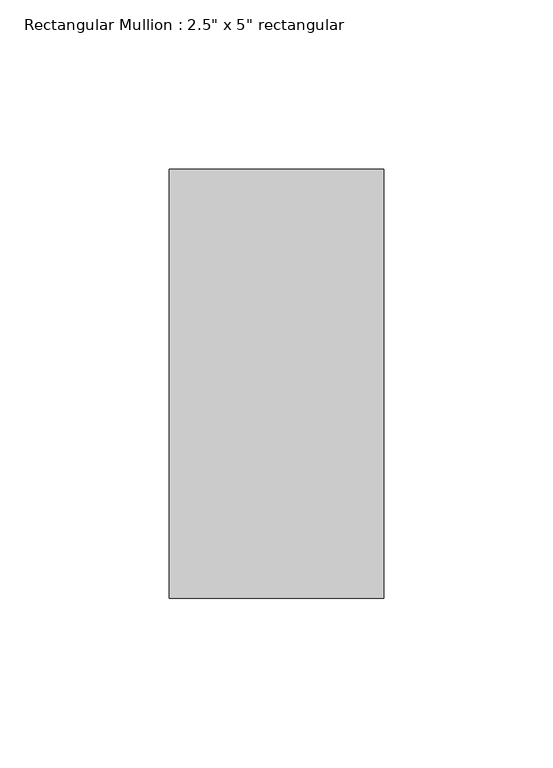
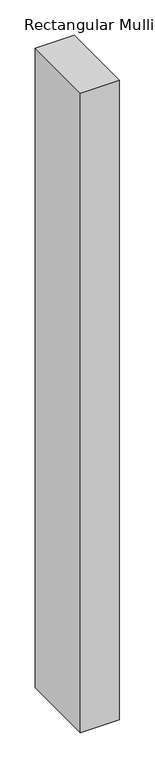
"""IFC4 building model written with IfcOpenShell, lengths in millimetres: member geometry."""

from ifc_helpers import new_model, si_unit, frame, origin, place, context, project, spatial, polyline, outline, extrude, source, transform, mapped, element, save


def member_c45b528a(model_context):
    return source(origin(), model_context, "Body", "SweptSolid", [
        extrude(outline(polyline([(31.75, 63.5), (31.75, -63.5), (-31.75, -63.5), (-31.75, 63.5), (31.75, 63.5)])), frame((0.0, 0.0, -1100.6666665), z_axis=(0.0, 0.0, 1.0), x_axis=(1.0, 0.0, 0.0)), (0.0, 0.0, 1.0), 1100.6666665),
    ])


if __name__ == "__main__":
    model = new_model("IFC4")
    model_context = context("Model", 3, world=origin())
    ifc_project = project(units=[si_unit("LENGTHUNIT", "METRE", prefix="MILLI")], contexts=[model_context])
    site = spatial("IfcSite", under=ifc_project)
    building = spatial("IfcBuilding", under=site)
    placement = place(None, origin())
    member_shape = member_c45b528a(model_context)
    element("IfcMember", 1, ObjectType="Rectangular Mullion : 2.5\" x 5\" rectangular", at=placement, inside=building, context=model_context, shape_type="MappedRepresentation", body=[
        mapped(member_shape, transform((0.0, 0.0, 0.0), x_axis=(1.0, 0.0, 0.0), y_axis=(0.0, 1.0, 0.0), z_axis=(0.0, 0.0, 1.0))),
    ])
    save(model, "model.ifc")

# Revit data of these elements
# Type "Rectangular Mullion : 2.5\" x 5\" rectangular"
#   built-in parameter 1007304 = 0.416667 (stored number, unit not read)
#   built-in parameter 1007301 = 0.104167 (stored number, unit not read)
#   built-in parameter 1007300 = 0.104167 (stored number, unit not read)
# Element 1 (IfcMember, "Rectangular Mullion : 2.5\" x 5\" rectangular")
#   Materials on its faces: "metal black"
# Materials
#   "metal black": class "Generic", colour RGB 120 120 120, transparency 0, Cost = 0
